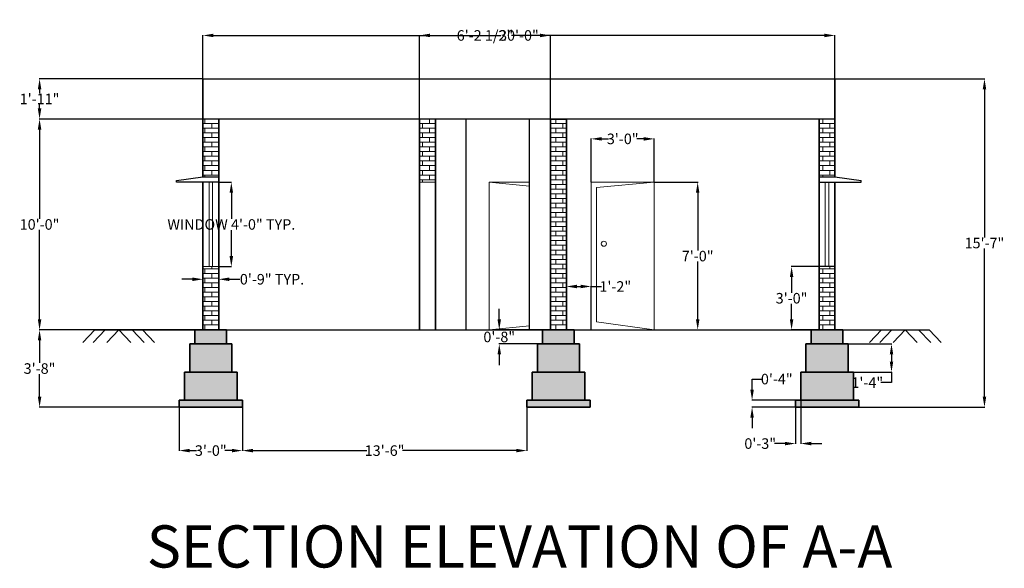
# Model space of a CAD drawing. Units: inches. Extents: x 94 to 277359, y -289541 to 1081.
# Tile 4 of 5: x 740 to 1300, y 353 to 665. Entities that reach past the tile are written whole.
import ezdxf

# ---------------------------------------------------------------- set-up
doc = ezdxf.new("R2010")
doc.units = ezdxf.units.IN
doc.header["$MEASUREMENT"] = 0
doc.layers.get('Defpoints').update_dxf_attribs({"color": 255})
for name, color, linetype, lineweight in [('A-ANNO-DIMS', 2, 'Continuous', 18), ('A-ANNO-TEXT', 7, 'Continuous', 30), ('A-DOOR', 4, 'Continuous', 18), ('A-ELEV', 7, 'Continuous', 25), ('A-ROOF', 7, 'Continuous', 30), ('A-SECT', 7, 'Continuous', 35), ('A-WALL-PATT', 252, 'Continuous', 13), ('C-TOPO', 8, 'Continuous', 25), ('S-FNDN', 7, 'Continuous', 35), ('S-FNDN-PATT', 252, 'Continuous', 13), ('window', 13, 'Continuous', 18)]:
    doc.layers.add(name, color=color, linetype=linetype, lineweight=lineweight)
doc.styles.get("Standard").update_dxf_attribs({"font": 'arial.ttf'})
doc.dimstyles.get("Standard").update_dxf_attribs({"dimtxt": 6, "dimasz": 6, "dimexe": 0.18, "dimexo": 0.0625, "dimgap": 0.09, "dimtad": 0, "dimtih": 1, "dimtoh": 1, "dimdec": 1, "dimzin": 0, "dimdsep": 46, "dimlunit": 3, "dimtxsty": 'Standard', "dimcen": 0.09, "dimadec": 0, "dimazin": 0, "dimtfac": 1, "dimtdec": 1, "dimtofl": 0, "dimtmove": 0, "dimatfit": 3, "dimfxl": 1, "dimtolj": 1, "dimtzin": 0, "dimarcsym": 0})
pattern_1 = [(50, (-239.0183, 16.959), (7.172602, -0.627521), [0.75, -8.25]), (355, (-239.018, 16.959), (-1.387513, 7.52192), [0.6, -6.6]), (100.45144, (-238.4206, 16.907), (5.78509, 6.8944), [0.637402, -7.01142]), (46.1842, (-239.018, 18.959), (10.672413, -1.655193), [1.125, -12.375]), (96.6356, (-238.129, 18.821), (9.34662, 9.741186), [0.9561, -10.51714]), (351.1842, (-239.018, 18.959), (9.34662, 9.741186), [0.9, -9.9]), (21, (-238.0183, 18.459), (5.96907, -4.02619), [0.75, -8.25]), (326, (-238.018, 18.459), (2.433153, 7.2515), [0.6, -6.6]), (71.45144, (-237.521, 18.124), (8.402224, 3.22531), [0.637402, -7.01142]), (37.5, (-239.0183, 16.9592), (0.1215986, 3.3289385), [0, -6.52, 0, -6.7, 0, -6.625]), (7.5, (-239.0183, 16.9592), (2.630695, 3.944117), [0, -3.82, 0, -6.37, 0, -2.525]), (327.5, (-241.2483, 16.9592), (5.3382244, -0.2255487), [0, -2.5, 0, -7.8, 0, -10.35]), (317.5, (-242.2483, 16.9592), (5.831862, 1.00105), [0, -3.25, 0, -5.18, 0, -7.35])]

# ---------------------------------------------------------------- blocks, each defined once
blk = doc.blocks.new('WE')
at = {"layer": 'window'}
for p, q in [((39.8, -77.7), (48.8, -77.7)), ((43.3, -77.7), (43.3, -125.7)), ((45.3, -77.7), (45.3, -125.7)), ((39.8, -125.7), (48.8, -125.7))]:
    blk.add_line(p, q, dxfattribs=at)
blk = doc.blocks.new('GRADE-MARK')
for p, q in [((6.85, 7.09), (0, 0)), ((12.76, 7.09), (5.91, 0)), ((20.39, 7.09), (13.54, 0)), ((20.39, 7.09), (27.24, 0)), ((28.01, 7.09), (34.86, 0)), ((33.93, 7.09), (40.78, 0))]:
    blk.add_line(p, q)
blk = doc.blocks.new('*D33')
at = {"layer": 'A-ANNO-DIMS', "color": 0, "lineweight": -2, "transparency": 16777216}
for p, q in [((853.01, 572.91), (860.33, 572.91)), ((860.15, 566.91), (860.15, 552.1)), ((860.15, 530.91), (860.15, 545.71)), ((853.01, 524.91), (860.33, 524.91))]:
    blk.add_line(p, q, dxfattribs=at)
at = {"layer": 'A-ANNO-DIMS', "color": 0, "transparency": 16777216}
for points in [[(859.15, 566.91), (861.15, 566.91), (860.15, 572.91)], [(859.15, 530.91), (861.15, 530.91), (860.15, 524.91)]]:
    blk.add_solid(points, dxfattribs=at)
at = {"layer": 'Defpoints', "color": 0, "transparency": 16777216}
for p in [(852.95, 572.91), (860.15, 572.91), (852.95, 524.91)]:
    blk.add_point(p, dxfattribs=at)
at = {"layer": 'A-ANNO-DIMS', "color": 0, "transparency": 16777216, "insert": (860.15, 548.91), "char_height": 6, "attachment_point": 5}
blk.add_mtext('\\A1;WINDOW 4\'-0" TYP.', dxfattribs=at)
blk = doc.blocks.new('*D34')
at = {"layer": 'A-ANNO-DIMS', "color": 0, "lineweight": -2, "transparency": 16777216}
for p, q in [((843.95, 524.84), (843.95, 517.53)), ((852.95, 524.84), (852.95, 517.53)), ((837.95, 517.71), (831.95, 517.71)), ((858.95, 517.71), (864.95, 517.71))]:
    blk.add_line(p, q, dxfattribs=at)
at = {"layer": 'A-ANNO-DIMS', "color": 0, "transparency": 16777216}
for points in [[(837.95, 518.71), (837.95, 516.71), (843.95, 517.71)], [(858.95, 518.71), (858.95, 516.71), (852.95, 517.71)]]:
    blk.add_solid(points, dxfattribs=at)
at = {"layer": 'Defpoints', "color": 0, "transparency": 16777216}
for p in [(843.95, 524.91), (852.95, 524.91), (852.95, 517.71)]:
    blk.add_point(p, dxfattribs=at)
at = {"layer": 'A-ANNO-DIMS', "color": 0, "transparency": 16777216, "insert": (883.32, 517.71), "char_height": 6, "attachment_point": 5}
blk.add_mtext('\\A1;0\'-9" TYP.', dxfattribs=at)
blk = doc.blocks.new('*D80')
at = {"layer": 'A-ANNO-DIMS', "color": 0, "lineweight": -2, "transparency": 16777216}
for p, q in [((843.95, 631.84), (843.95, 656.65)), ((849.95, 656.47), (1013.55, 656.47)), ((1197.95, 656.47), (1034.34, 656.47)), ((1203.95, 631.84), (1203.95, 656.65))]:
    blk.add_line(p, q, dxfattribs=at)
at = {"layer": 'A-ANNO-DIMS', "color": 0, "transparency": 16777216}
for points in [[(849.95, 657.47), (849.95, 655.47), (843.95, 656.47)], [(1197.95, 657.47), (1197.95, 655.47), (1203.95, 656.47)]]:
    blk.add_solid(points, dxfattribs=at)
at = {"layer": 'Defpoints', "color": 0, "transparency": 16777216}
for p in [(1203.95, 656.47), (843.95, 631.77), (1203.95, 631.77)]:
    blk.add_point(p, dxfattribs=at)
at = {"layer": 'A-ANNO-DIMS', "color": 0, "transparency": 16777216, "insert": (1023.95, 656.47), "char_height": 6, "attachment_point": 5}
blk.add_mtext('\\A1;30\'-0"', dxfattribs=at)
blk = doc.blocks.new('*D81')
at = {"layer": 'A-ANNO-DIMS', "color": 0, "lineweight": -2, "transparency": 16777216}
for p, q in [((1204.01, 631.77), (1289.27, 631.77)), ((1289.09, 625.77), (1289.09, 541.49)), ((1289.09, 450.91), (1289.09, 535.19)), ((1217.51, 444.91), (1289.27, 444.91))]:
    blk.add_line(p, q, dxfattribs=at)
at = {"layer": 'A-ANNO-DIMS', "color": 0, "transparency": 16777216}
for points in [[(1288.09, 625.77), (1290.09, 625.77), (1289.09, 631.77)], [(1288.09, 450.91), (1290.09, 450.91), (1289.09, 444.91)]]:
    blk.add_solid(points, dxfattribs=at)
at = {"layer": 'Defpoints', "color": 0, "transparency": 16777216}
for p in [(1203.95, 631.77), (1289.09, 631.77), (1217.45, 444.91)]:
    blk.add_point(p, dxfattribs=at)
at = {"layer": 'A-ANNO-DIMS', "color": 0, "transparency": 16777216, "insert": (1289.09, 538.34), "char_height": 6, "attachment_point": 5}
blk.add_mtext('\\A1;15\'-7"', dxfattribs=at)
blk = doc.blocks.new('*D82')
at = {"layer": 'A-ANNO-DIMS', "color": 0, "lineweight": -2, "transparency": 16777216}
for p, q in [((843.89, 608.91), (750.74, 608.91)), ((750.92, 602.91), (750.92, 552.06)), ((750.92, 494.91), (750.92, 545.75)), ((843.89, 488.91), (750.74, 488.91))]:
    blk.add_line(p, q, dxfattribs=at)
at = {"layer": 'A-ANNO-DIMS', "color": 0, "transparency": 16777216}
for points in [[(749.92, 602.91), (751.92, 602.91), (750.92, 608.91)], [(749.92, 494.91), (751.92, 494.91), (750.92, 488.91)]]:
    blk.add_solid(points, dxfattribs=at)
at = {"layer": 'Defpoints', "color": 0, "transparency": 16777216}
for p in [(750.92, 608.91), (843.95, 608.91), (843.95, 488.91)]:
    blk.add_point(p, dxfattribs=at)
at = {"layer": 'A-ANNO-DIMS', "color": 0, "transparency": 16777216, "insert": (750.92, 548.91), "char_height": 6, "attachment_point": 5}
blk.add_mtext('\\A1;10\'-0"', dxfattribs=at)
blk = doc.blocks.new('*D83')
at = {"layer": 'A-ANNO-DIMS', "color": 0, "lineweight": -2, "transparency": 16777216}
for p, q in [((839.39, 488.91), (750.74, 488.91)), ((750.92, 482.91), (750.92, 470.06)), ((750.92, 450.91), (750.92, 463.75)), ((830.39, 444.91), (750.74, 444.91))]:
    blk.add_line(p, q, dxfattribs=at)
at = {"layer": 'A-ANNO-DIMS', "color": 0, "transparency": 16777216}
for points in [[(749.92, 482.91), (751.92, 482.91), (750.92, 488.91)], [(749.92, 450.91), (751.92, 450.91), (750.92, 444.91)]]:
    blk.add_solid(points, dxfattribs=at)
at = {"layer": 'Defpoints', "color": 0, "transparency": 16777216}
for p in [(750.92, 488.91), (839.45, 488.91), (830.45, 444.91)]:
    blk.add_point(p, dxfattribs=at)
at = {"layer": 'A-ANNO-DIMS', "color": 0, "transparency": 16777216, "insert": (750.92, 466.91), "char_height": 6, "attachment_point": 5}
blk.add_mtext('\\A1;3\'-8"', dxfattribs=at)
blk = doc.blocks.new('*D84')
at = {"layer": 'A-ANNO-DIMS', "color": 0, "lineweight": -2, "transparency": 16777216}
for p, q in [((843.89, 631.77), (750.74, 631.77)), ((750.92, 625.77), (750.92, 623.44)), ((750.92, 614.91), (750.92, 617.24)), ((843.89, 608.91), (750.74, 608.91))]:
    blk.add_line(p, q, dxfattribs=at)
at = {"layer": 'A-ANNO-DIMS', "color": 0, "transparency": 16777216}
for points in [[(749.92, 625.77), (751.92, 625.77), (750.92, 631.77)], [(749.92, 614.91), (751.92, 614.91), (750.92, 608.91)]]:
    blk.add_solid(points, dxfattribs=at)
at = {"layer": 'Defpoints', "color": 0, "transparency": 16777216}
for p in [(750.92, 631.77), (843.95, 631.77), (843.95, 608.91)]:
    blk.add_point(p, dxfattribs=at)
at = {"layer": 'A-ANNO-DIMS', "color": 0, "transparency": 16777216, "insert": (750.92, 620.34), "char_height": 6, "attachment_point": 5}
blk.add_mtext('\\A1;1\'-11"', dxfattribs=at)
blk = doc.blocks.new('*D85')
at = {"layer": 'A-ANNO-DIMS', "color": 0, "lineweight": -2, "transparency": 16777216}
for p, q in [((830.45, 444.84), (830.45, 420.03)), ((866.45, 444.84), (866.45, 420.03)), ((836.45, 420.21), (840.39, 420.21)), ((860.45, 420.21), (856.51, 420.21))]:
    blk.add_line(p, q, dxfattribs=at)
at = {"layer": 'A-ANNO-DIMS', "color": 0, "transparency": 16777216}
for points in [[(836.45, 421.21), (836.45, 419.21), (830.45, 420.21)], [(860.45, 421.21), (860.45, 419.21), (866.45, 420.21)]]:
    blk.add_solid(points, dxfattribs=at)
at = {"layer": 'Defpoints', "color": 0, "transparency": 16777216}
for p in [(830.45, 444.91), (866.45, 444.91), (866.45, 420.21)]:
    blk.add_point(p, dxfattribs=at)
at = {"layer": 'A-ANNO-DIMS', "color": 0, "transparency": 16777216, "insert": (848.45, 420.21), "char_height": 6, "attachment_point": 5}
blk.add_mtext('\\A1;3\'-0"', dxfattribs=at)
blk = doc.blocks.new('*D86')
at = {"layer": 'A-ANNO-DIMS', "color": 0, "lineweight": -2, "transparency": 16777216}
for p, q in [((866.45, 444.84), (866.45, 420.03)), ((1028.45, 444.84), (1028.45, 420.03)), ((872.45, 420.21), (937.33, 420.21)), ((1022.45, 420.21), (957.56, 420.21))]:
    blk.add_line(p, q, dxfattribs=at)
at = {"layer": 'A-ANNO-DIMS', "color": 0, "transparency": 16777216}
for points in [[(872.45, 421.21), (872.45, 419.21), (866.45, 420.21)], [(1022.45, 421.21), (1022.45, 419.21), (1028.45, 420.21)]]:
    blk.add_solid(points, dxfattribs=at)
at = {"layer": 'Defpoints', "color": 0, "transparency": 16777216}
for p in [(866.45, 444.91), (1028.45, 444.91), (1028.45, 420.21)]:
    blk.add_point(p, dxfattribs=at)
at = {"layer": 'A-ANNO-DIMS', "color": 0, "transparency": 16777216, "insert": (947.45, 420.21), "char_height": 6, "attachment_point": 5}
blk.add_mtext('\\A1;13\'-6"', dxfattribs=at)
blk = doc.blocks.new('*D87')
at = {"layer": 'A-ANNO-DIMS', "color": 0, "lineweight": -2, "transparency": 16777216}
for p, q in [((967.32, 608.97), (967.32, 656.65)), ((973.32, 656.47), (989.56, 656.47)), ((1035.95, 656.47), (1019.7, 656.47)), ((1041.95, 608.97), (1041.95, 656.65))]:
    blk.add_line(p, q, dxfattribs=at)
at = {"layer": 'A-ANNO-DIMS', "color": 0, "transparency": 16777216}
for points in [[(973.32, 657.47), (973.32, 655.47), (967.32, 656.47)], [(1035.95, 657.47), (1035.95, 655.47), (1041.95, 656.47)]]:
    blk.add_solid(points, dxfattribs=at)
at = {"layer": 'Defpoints', "color": 0, "transparency": 16777216}
for p in [(1041.95, 656.47), (967.32, 608.91), (1041.95, 608.91)]:
    blk.add_point(p, dxfattribs=at)
at = {"layer": 'A-ANNO-DIMS', "color": 0, "transparency": 16777216, "insert": (1004.63, 656.47), "char_height": 6, "attachment_point": 5}
blk.add_mtext('\\A1;6\'-2 1/2"', dxfattribs=at)
blk = doc.blocks.new('*D88')
at = {"layer": 'A-ANNO-DIMS', "color": 0, "lineweight": -2, "transparency": 16777216}
for p, q in [((1101.13, 572.91), (1125.94, 572.91)), ((1125.76, 566.91), (1125.76, 534.06)), ((1125.76, 494.91), (1125.76, 527.75)), ((1101.13, 488.91), (1125.94, 488.91))]:
    blk.add_line(p, q, dxfattribs=at)
at = {"layer": 'A-ANNO-DIMS', "color": 0, "transparency": 16777216}
for points in [[(1124.76, 566.91), (1126.76, 566.91), (1125.76, 572.91)], [(1124.76, 494.91), (1126.76, 494.91), (1125.76, 488.91)]]:
    blk.add_solid(points, dxfattribs=at)
at = {"layer": 'Defpoints', "color": 0, "transparency": 16777216}
for p in [(1101.06, 572.91), (1101.06, 488.91), (1125.76, 488.91)]:
    blk.add_point(p, dxfattribs=at)
at = {"layer": 'A-ANNO-DIMS', "color": 0, "transparency": 16777216, "insert": (1125.76, 530.91), "char_height": 6, "attachment_point": 5}
blk.add_mtext('\\A1;7\'-0"', dxfattribs=at)
blk = doc.blocks.new('*D89')
at = {"layer": 'A-ANNO-DIMS', "color": 0, "lineweight": -2, "transparency": 16777216}
for p, q in [((1065.06, 572.97), (1065.06, 597.79)), ((1071.06, 597.61), (1075, 597.61)), ((1095.06, 597.61), (1091.13, 597.61)), ((1101.06, 572.97), (1101.06, 597.79))]:
    blk.add_line(p, q, dxfattribs=at)
at = {"layer": 'A-ANNO-DIMS', "color": 0, "transparency": 16777216}
for points in [[(1071.06, 598.61), (1071.06, 596.61), (1065.06, 597.61)], [(1095.06, 598.61), (1095.06, 596.61), (1101.06, 597.61)]]:
    blk.add_solid(points, dxfattribs=at)
at = {"layer": 'Defpoints', "color": 0, "transparency": 16777216}
for p in [(1101.06, 597.61), (1065.06, 572.91), (1101.06, 572.91)]:
    blk.add_point(p, dxfattribs=at)
at = {"layer": 'A-ANNO-DIMS', "color": 0, "transparency": 16777216, "insert": (1083.06, 597.61), "char_height": 6, "attachment_point": 5}
blk.add_mtext('\\A1;3\'-0"', dxfattribs=at)
blk = doc.blocks.new('*D90')
at = {"layer": 'A-ANNO-DIMS', "color": 0, "lineweight": -2, "transparency": 16777216}
for p, q in [((1203.89, 524.91), (1179.07, 524.91)), ((1179.25, 518.91), (1179.25, 510.06)), ((1179.25, 494.91), (1179.25, 503.75)), ((1203.89, 488.91), (1179.07, 488.91))]:
    blk.add_line(p, q, dxfattribs=at)
at = {"layer": 'A-ANNO-DIMS', "color": 0, "transparency": 16777216}
for points in [[(1178.25, 518.91), (1180.25, 518.91), (1179.25, 524.91)], [(1178.25, 494.91), (1180.25, 494.91), (1179.25, 488.91)]]:
    blk.add_solid(points, dxfattribs=at)
at = {"layer": 'Defpoints', "color": 0, "transparency": 16777216}
for p in [(1179.25, 524.91), (1203.95, 524.91), (1203.95, 488.91)]:
    blk.add_point(p, dxfattribs=at)
at = {"layer": 'A-ANNO-DIMS', "color": 0, "transparency": 16777216, "insert": (1179.25, 506.91), "char_height": 6, "attachment_point": 5}
blk.add_mtext('\\A1;3\'-0"', dxfattribs=at)
blk = doc.blocks.new('*D91')
at = {"layer": 'A-ANNO-DIMS', "color": 0, "lineweight": -2, "transparency": 16777216}
for p, q in [((1050.95, 488.97), (1050.95, 513.79)), ((1056.95, 513.61), (1059.06, 513.61)), ((1065.06, 488.97), (1065.06, 513.79)), ((1065.06, 513.61), (1071.06, 513.61))]:
    blk.add_line(p, q, dxfattribs=at)
at = {"layer": 'A-ANNO-DIMS', "color": 0, "transparency": 16777216}
for points in [[(1056.95, 514.61), (1056.95, 512.61), (1050.95, 513.61)], [(1059.06, 514.61), (1059.06, 512.61), (1065.06, 513.61)]]:
    blk.add_solid(points, dxfattribs=at)
at = {"layer": 'Defpoints', "color": 0, "transparency": 16777216}
for p in [(1065.06, 513.61), (1050.95, 488.91), (1065.06, 488.91)]:
    blk.add_point(p, dxfattribs=at)
at = {"layer": 'A-ANNO-DIMS', "color": 0, "transparency": 16777216, "insert": (1078.85, 513.61), "char_height": 6, "attachment_point": 5}
blk.add_mtext('\\A1;1\'-2"', dxfattribs=at)
blk = doc.blocks.new('*D92')
at = {"layer": 'A-ANNO-DIMS', "color": 0, "lineweight": -2, "transparency": 16777216}
for p, q in [((1012.747749, 494.905028), (1012.747749, 500.905028)), ((1037.385249, 488.905028), (1012.567749, 488.905028)), ((1037.385249, 480.905028), (1012.567749, 480.905028)), ((1012.747749, 474.905028), (1012.747749, 468.905028))]:
    blk.add_line(p, q, dxfattribs=at)
at = {"layer": 'A-ANNO-DIMS', "color": 0, "transparency": 16777216}
for points in [[(1011.747749, 494.905028), (1013.747749, 494.905028), (1012.747749, 488.905028)], [(1011.747749, 474.905028), (1013.747749, 474.905028), (1012.747749, 480.905028)]]:
    blk.add_solid(points, dxfattribs=at)
at = {"layer": 'Defpoints', "color": 0, "transparency": 16777216}
for p in [(1012.747749, 488.905028), (1037.447749, 488.905028), (1037.447749, 480.905028)]:
    blk.add_point(p, dxfattribs=at)
at = {"layer": 'A-ANNO-DIMS', "color": 0, "transparency": 16777216, "insert": (1012.747749, 484.905028), "char_height": 6, "attachment_point": 5}
blk.add_mtext('\\A1;0\'-8"', dxfattribs=at)
blk = doc.blocks.new('*D93')
at = {"layer": 'A-ANNO-DIMS', "color": 0, "lineweight": -2, "transparency": 16777216}
for p, q in [((1211.51, 480.91), (1236.33, 480.91)), ((1236.15, 474.91), (1236.15, 470.91)), ((1211.51, 464.91), (1236.33, 464.91)), ((1236.15, 464.91), (1236.15, 458.91)), ((1236.15, 458.91), (1230.15, 458.91))]:
    blk.add_line(p, q, dxfattribs=at)
at = {"layer": 'A-ANNO-DIMS', "color": 0, "transparency": 16777216}
for points in [[(1235.15, 474.91), (1237.15, 474.91), (1236.15, 480.91)], [(1235.15, 470.91), (1237.15, 470.91), (1236.15, 464.91)]]:
    blk.add_solid(points, dxfattribs=at)
at = {"layer": 'Defpoints', "color": 0, "transparency": 16777216}
for p in [(1211.45, 480.91), (1211.45, 464.91), (1236.15, 464.91)]:
    blk.add_point(p, dxfattribs=at)
at = {"layer": 'A-ANNO-DIMS', "color": 0, "transparency": 16777216, "insert": (1222.37, 458.91), "char_height": 6, "attachment_point": 5}
blk.add_mtext('\\A1;1\'-4"', dxfattribs=at)
blk = doc.blocks.new('*D94')
at = {"layer": 'A-ANNO-DIMS', "color": 0, "lineweight": -2, "transparency": 16777216}
for p, q in [((1181.45, 448.84), (1181.45, 424.03)), ((1184.45, 448.84), (1184.45, 424.03)), ((1175.45, 424.21), (1169.45, 424.21)), ((1190.45, 424.21), (1196.45, 424.21))]:
    blk.add_line(p, q, dxfattribs=at)
at = {"layer": 'A-ANNO-DIMS', "color": 0, "transparency": 16777216}
for points in [[(1175.45, 425.21), (1175.45, 423.21), (1181.45, 424.21)], [(1190.45, 425.21), (1190.45, 423.21), (1184.45, 424.21)]]:
    blk.add_solid(points, dxfattribs=at)
at = {"layer": 'Defpoints', "color": 0, "transparency": 16777216}
for p in [(1181.45, 448.91), (1184.45, 448.91), (1181.45, 424.21)]:
    blk.add_point(p, dxfattribs=at)
at = {"layer": 'A-ANNO-DIMS', "color": 0, "transparency": 16777216, "insert": (1161.38, 424.21), "char_height": 6, "attachment_point": 5}
blk.add_mtext('\\A1;0\'-3"', dxfattribs=at)
blk = doc.blocks.new('*D95')
at = {"layer": 'A-ANNO-DIMS', "color": 0, "lineweight": -2, "transparency": 16777216}
for p, q in [((1156.75, 454.91), (1156.75, 460.91)), ((1156.75, 460.91), (1162.75, 460.91)), ((1181.39, 448.91), (1156.57, 448.91)), ((1181.39, 444.91), (1156.57, 444.91)), ((1156.75, 438.91), (1156.75, 432.91))]:
    blk.add_line(p, q, dxfattribs=at)
at = {"layer": 'A-ANNO-DIMS', "color": 0, "transparency": 16777216}
for points in [[(1155.75, 454.91), (1157.75, 454.91), (1156.75, 448.91)], [(1155.75, 438.91), (1157.75, 438.91), (1156.75, 444.91)]]:
    blk.add_solid(points, dxfattribs=at)
at = {"layer": 'Defpoints', "color": 0, "transparency": 16777216}
for p in [(1156.75, 448.91), (1181.45, 448.91), (1181.45, 444.91)]:
    blk.add_point(p, dxfattribs=at)
at = {"layer": 'A-ANNO-DIMS', "color": 0, "transparency": 16777216, "insert": (1170.81, 460.91), "char_height": 6, "attachment_point": 5}
blk.add_mtext('\\A1;0\'-4"', dxfattribs=at)

msp = doc.modelspace()

# ---------------------------------------------------------------- hatches: boundary and pattern name
at = {"layer": 'A-WALL-PATT'}
h = msp.add_hatch(dxfattribs=at)
h.set_pattern_fill('AR-BRSTD', color=256)
h.set_pattern_definition([(0, (-239.0183, 16.9592), (0, 2.667), []), (90, (-239.0183, 16.9592), (-4, 2.667), [2.667, -2.667])])
h.paths.add_polyline_path([(852.95, 608.91), (843.95, 608.91), (843.95, 575.91), (852.95, 575.91)])
h.paths.add_polyline_path([(852.95, 524.91), (843.95, 524.91), (843.95, 488.91), (848.45, 488.91), (852.95, 488.91)])
h.paths.add_polyline_path([(976.4, 608.91), (967.32, 608.91), (967.32, 572.91), (976.4, 572.91)])
h.paths.add_polyline_path([(1041.95, 488.91), (1046.45, 488.91), (1050.95, 488.91), (1050.95, 608.91), (1041.95, 608.91)])
h.paths.add_polyline_path([(1194.95, 575.91), (1203.95, 575.91), (1203.95, 608.91), (1194.95, 608.91)])
h.paths.add_polyline_path([(1203.95, 524.91), (1194.95, 524.91), (1194.95, 488.91), (1199.45, 488.91), (1203.95, 488.91)])
at = {"layer": 'S-FNDN-PATT'}
h = msp.add_hatch(dxfattribs=at)
h.set_pattern_fill('AR-CONC', color=256)
h.set_pattern_definition(pattern_1)
h.paths.add_polyline_path([(848.45, 480.91), (857.45, 480.91), (857.45, 488.91), (848.45, 488.91), (839.45, 488.91), (839.45, 480.91)])
h.paths.add_polyline_path([(1055.45, 480.91), (1055.45, 488.91), (1046.45, 488.91), (1037.45, 488.91), (1037.45, 480.91), (1046.45, 480.91)])
h.paths.add_polyline_path([(1199.45, 480.91), (1208.45, 480.91), (1208.45, 488.91), (1199.45, 488.91), (1190.45, 488.91), (1190.45, 480.91)])
h = msp.add_hatch(dxfattribs=at)
h.set_pattern_fill('ANSI33', color=256, scale=10)
h.set_pattern_definition([(45, (-239.0183, 16.9592), (-1.767767, 1.767767), []), (45, (-237.2506, 16.9592), (-1.767767, 1.767767), [1.25, -0.625])])
h.paths.add_polyline_path([(863.45, 464.91), (848.45, 464.91), (836.45, 464.91), (833.45, 464.91), (833.45, 448.91), (848.45, 448.91), (863.45, 448.91)])
h.paths.add_polyline_path([(860.45, 480.91), (848.45, 480.91), (839.45, 480.91), (836.45, 480.91), (836.45, 464.91), (848.45, 464.91), (860.45, 464.91)])
h.paths.add_polyline_path([(1061.45, 464.91), (1046.45, 464.91), (1034.45, 464.91), (1031.45, 464.91), (1031.45, 448.91), (1046.45, 448.91), (1061.45, 448.91)])
h.paths.add_polyline_path([(1058.45, 480.91), (1046.45, 480.91), (1037.45, 480.91), (1034.45, 480.91), (1034.45, 464.91), (1046.45, 464.91), (1058.45, 464.91)])
h.paths.add_polyline_path([(1214.45, 464.91), (1199.45, 464.91), (1187.45, 464.91), (1184.45, 464.91), (1184.45, 448.91), (1199.45, 448.91), (1214.45, 448.91)])
h.paths.add_polyline_path([(1211.45, 480.91), (1199.45, 480.91), (1190.45, 480.91), (1187.45, 480.91), (1187.45, 464.91), (1199.45, 464.91), (1211.45, 464.91)])
h = msp.add_hatch(dxfattribs=at)
h.set_pattern_fill('AR-CONC', color=256)
h.set_pattern_definition(pattern_1)
h.paths.add_polyline_path([(866.45, 444.91), (866.45, 448.91), (848.45, 448.91), (833.45, 448.91), (830.45, 448.91), (830.45, 444.91)])
h.paths.add_polyline_path([(1064.45, 448.91), (1046.45, 448.91), (1031.45, 448.91), (1028.45, 448.91), (1028.45, 444.91), (1064.45, 444.91)])
h.paths.add_polyline_path([(1217.45, 444.91), (1217.45, 448.91), (1199.45, 448.91), (1184.45, 448.91), (1181.45, 448.91), (1181.45, 444.91)])

# ---------------------------------------------------------------- linework, layer by layer
at = {"layer": 'A-DOOR'}
for p, q in [((976.4, 572.91), (967.32, 572.91)), ((976.4, 488.91), (976.4, 572.91)), ((1006.95, 488.91), (1006.95, 572.91)), ((1006.95, 572.91), (1029.95, 572.91)), ((1006.95, 572.91), (1029.95, 570.71)), ((1065.06, 488.91), (1065.06, 572.91)), ((1065.06, 572.91), (1101.06, 572.91)), ((1101.06, 572.91), (1068.16, 569.94)), ((1101.06, 572.91), (1101.06, 488.91)), ((1068.16, 569.94), (1068.16, 493.45)), ((1006.95, 488.91), (1029.95, 491.24)), ((1068.16, 493.45), (1101.06, 488.91))]:
    msp.add_line(p, q, dxfattribs=at)
msp.add_circle((1072.34, 537.94), 1.47, dxfattribs=at)
at = {"layer": 'A-ELEV'}
for p, q in [((993.95, 488.91), (993.95, 608.91)), ((1029.95, 488.91), (1029.95, 608.91))]:
    msp.add_line(p, q, dxfattribs=at)
at = {"layer": 'A-ROOF'}
for p, q in [((843.95, 631.77), (1203.95, 631.77)), ((1203.95, 608.91), (843.95, 608.91)), ((828.95, 573.91), (843.95, 575.91)), ((828.95, 572.91), (828.95, 573.91)), ((852.95, 572.91), (828.95, 572.91)), ((843.95, 575.91), (852.95, 575.91)), ((1194.95, 572.91), (1194.95, 575.91)), ((1194.95, 575.91), (1203.95, 575.91)), ((1194.95, 572.91), (1218.95, 572.91)), ((1203.95, 575.91), (1218.95, 573.91)), ((1218.95, 572.91), (1218.95, 573.91))]:
    msp.add_line(p, q, dxfattribs=at)
at = {"layer": 'A-SECT'}
for p, q in [((843.95, 575.91), (843.95, 631.77)), ((1203.95, 575.91), (1203.95, 631.77)), ((852.95, 608.91), (852.95, 488.91)), ((967.32, 488.91), (967.32, 608.91)), ((976.4, 488.91), (976.4, 608.91)), ((1041.95, 488.91), (1041.95, 608.91)), ((1041.95, 608.91), (1050.95, 608.91)), ((1050.95, 608.91), (1050.95, 488.91)), ((1194.95, 488.91), (1194.95, 608.91)), ((843.95, 488.91), (843.95, 572.91)), ((1203.95, 488.91), (1203.95, 572.91)), ((843.95, 488.91), (852.95, 488.91)), ((1041.95, 488.91), (1050.95, 488.91)), ((1194.95, 488.91), (1203.95, 488.91))]:
    msp.add_line(p, q, dxfattribs=at)
at = {"layer": 'C-TOPO'}
msp.add_line((782.46, 488.91), (1257.54, 488.91), dxfattribs=at)
at = {"layer": 'S-FNDN'}
for p, q in [((839.45, 480.91), (839.45, 488.91)), ((839.45, 488.91), (848.45, 488.91)), ((857.45, 488.91), (848.45, 488.91)), ((857.45, 480.91), (857.45, 488.91)), ((1037.45, 480.91), (1037.45, 488.91)), ((1037.45, 488.91), (1046.45, 488.91)), ((1055.45, 488.91), (1046.45, 488.91)), ((1055.45, 480.91), (1055.45, 488.91)), ((1190.45, 480.91), (1190.45, 488.91)), ((1190.45, 488.91), (1199.45, 488.91)), ((1208.45, 488.91), (1199.45, 488.91)), ((1208.45, 480.91), (1208.45, 488.91)), ((836.45, 464.91), (836.45, 480.91)), ((836.45, 480.91), (848.45, 480.91)), ((848.45, 480.91), (839.45, 480.91)), ((860.45, 480.91), (848.45, 480.91)), ((848.45, 480.91), (857.45, 480.91)), ((860.45, 464.91), (860.45, 480.91)), ((1034.45, 464.91), (1034.45, 480.91)), ((1034.45, 480.91), (1046.45, 480.91)), ((1046.45, 480.91), (1037.45, 480.91)), ((1058.45, 480.91), (1046.45, 480.91)), ((1046.45, 480.91), (1055.45, 480.91)), ((1058.45, 464.91), (1058.45, 480.91)), ((1187.45, 464.91), (1187.45, 480.91)), ((1187.45, 480.91), (1199.45, 480.91)), ((1199.45, 480.91), (1190.45, 480.91)), ((1211.45, 480.91), (1199.45, 480.91)), ((1199.45, 480.91), (1208.45, 480.91)), ((1211.45, 464.91), (1211.45, 480.91)), ((833.45, 448.91), (833.45, 464.91)), ((833.45, 464.91), (848.45, 464.91)), ((848.45, 464.91), (836.45, 464.91)), ((863.45, 464.91), (848.45, 464.91)), ((848.45, 464.91), (860.45, 464.91)), ((863.45, 448.91), (863.45, 464.91)), ((1031.45, 448.91), (1031.45, 464.91)), ((1031.45, 464.91), (1046.45, 464.91)), ((1046.45, 464.91), (1034.45, 464.91)), ((1061.45, 464.91), (1046.45, 464.91)), ((1046.45, 464.91), (1058.45, 464.91)), ((1061.45, 448.91), (1061.45, 464.91)), ((1184.45, 448.91), (1184.45, 464.91)), ((1184.45, 464.91), (1199.45, 464.91)), ((1199.45, 464.91), (1187.45, 464.91)), ((1214.45, 464.91), (1199.45, 464.91)), ((1199.45, 464.91), (1211.45, 464.91)), ((1214.45, 448.91), (1214.45, 464.91)), ((830.45, 444.91), (830.45, 448.91)), ((830.45, 448.91), (848.45, 448.91)), ((848.45, 448.91), (833.45, 448.91)), ((866.45, 448.91), (848.45, 448.91)), ((848.45, 448.91), (863.45, 448.91)), ((866.45, 444.91), (866.45, 448.91)), ((1028.45, 444.91), (1028.45, 448.91)), ((1028.45, 448.91), (1046.45, 448.91)), ((1046.45, 448.91), (1031.45, 448.91)), ((1064.45, 448.91), (1046.45, 448.91)), ((1046.45, 448.91), (1061.45, 448.91)), ((1064.45, 444.91), (1064.45, 448.91)), ((1181.45, 444.91), (1181.45, 448.91)), ((1181.45, 448.91), (1199.45, 448.91)), ((1199.45, 448.91), (1184.45, 448.91)), ((1217.45, 448.91), (1199.45, 448.91)), ((1199.45, 448.91), (1214.45, 448.91)), ((1217.45, 444.91), (1217.45, 448.91)), ((830.45, 444.91), (866.45, 444.91)), ((866.45, 444.91), (830.45, 444.91)), ((1028.45, 444.91), (1064.45, 444.91)), ((1064.45, 444.91), (1028.45, 444.91)), ((1181.45, 444.91), (1217.45, 444.91)), ((1217.45, 444.91), (1181.45, 444.91))]:
    msp.add_line(p, q, dxfattribs=at)

# ---------------------------------------------------------------- block references
at = {"layer": 'C-TOPO'}
for p in [(775.62, 481.81), (1223.61, 481.81)]:
    msp.add_blockref('GRADE-MARK', p, dxfattribs=at)
at = {"layer": 'window'}
for p in [(804.15, 650.61), (1155.15, 650.61)]:
    msp.add_blockref('WE', p, dxfattribs=at)

# ---------------------------------------------------------------- texts
at = {"layer": 'A-ANNO-TEXT', "insert": (1024.31, 377.66), "char_height": 24, "attachment_point": 2}
msp.add_mtext_dynamic_manual_height_columns('SECTION ELEVATION OF A-A ', width=589.888, gutter_width=1, heights=[0], dxfattribs=at)

# ---------------------------------------------------------------- dimensions: what is measured, and where the dimension line sits
at = {"layer": 'A-ANNO-DIMS'}
for base, p1, p2, picture, middle in [((1041.95, 656.47), (967.32, 608.91), (1041.95, 608.91), '*D87', (1004.63, 656.47)), ((1203.95, 656.47), (843.95, 631.77), (1203.95, 631.77), '*D80', (1023.95, 656.47)), ((1101.06, 597.61), (1065.06, 572.91), (1101.06, 572.91), '*D89', (1083.06, 597.61)), ((1065.06, 513.61), (1050.95, 488.91), (1065.06, 488.91), '*D91', (1078.85, 513.61)), ((866.45, 420.21), (830.45, 444.91), (866.45, 444.91), '*D85', (848.45, 420.21)), ((1028.45, 420.21), (866.45, 444.91), (1028.45, 444.91), '*D86', (947.45, 420.21))]:
    dim = msp.add_linear_dim(base=base, p1=p1, p2=p2, dimstyle='Standard', override={"dimdec": 1, "dimlfac": 1, "dimrnd": 0, "dimzin": 1, "dimdsep": 46, "dimlunit": 4, "dimfrac": 2}, dxfattribs=at)
    dim.commit()
    dim.dimension.update_dxf_attribs({"geometry": picture, "text_midpoint": middle})
for base, p1, p2, angle, picture, middle in [((750.92, 631.77), (843.95, 608.91), (843.95, 631.77), 90, '*D84', (750.92, 620.34)), ((1289.09, 631.77), (1217.45, 444.91), (1203.95, 631.77), 90, '*D81', (1289.09, 538.34)), ((750.92, 608.91), (843.95, 488.91), (843.95, 608.91), 90, '*D82', (750.92, 548.91)), ((1125.76, 488.91), (1101.06, 572.91), (1101.06, 488.91), 270, '*D88', (1125.76, 530.91)), ((1179.25, 524.91), (1203.95, 488.91), (1203.95, 524.91), 90, '*D90', (1179.25, 506.91)), ((1012.75, 488.91), (1037.45, 480.91), (1037.45, 488.91), 90, '*D92', (1012.75, 484.91)), ((750.92, 488.91), (830.45, 444.91), (839.45, 488.91), 90, '*D83', (750.92, 466.91)), ((1236.15, 464.91), (1211.45, 480.91), (1211.45, 464.91), 270, '*D93', (1222.37, 458.91)), ((1156.75, 448.91), (1181.45, 444.91), (1181.45, 448.91), 90, '*D95', (1170.81, 460.91)), ((1181.45, 424.21), (1184.45, 448.91), (1181.45, 448.91), 180, '*D94', (1161.38, 424.21))]:
    dim = msp.add_linear_dim(base=base, p1=p1, p2=p2, angle=angle, dimstyle='Standard', override={"dimdec": 1, "dimlfac": 1, "dimrnd": 0, "dimzin": 1, "dimdsep": 46, "dimlunit": 4, "dimfrac": 2}, dxfattribs=at)
    dim.commit()
    dim.dimension.update_dxf_attribs({"geometry": picture, "text_midpoint": middle})
dim = msp.add_linear_dim(base=(860.15, 572.91), p1=(852.95, 524.91), p2=(852.95, 572.91), angle=90, text='WINDOW <> TYP.', dimstyle='Standard', override={"dimdec": 1, "dimlfac": 1, "dimrnd": 0, "dimzin": 1, "dimdsep": 46, "dimlunit": 4, "dimfrac": 2}, dxfattribs=at)
dim.commit()
dim.dimension.update_dxf_attribs({"geometry": '*D33', "text_midpoint": (860.15, 548.91)})
dim = msp.add_linear_dim(base=(852.95, 517.71), p1=(843.95, 524.91), p2=(852.95, 524.91), text='<> TYP.', dimstyle='Standard', override={"dimdec": 1, "dimlfac": 1, "dimrnd": 0, "dimzin": 1, "dimdsep": 46, "dimlunit": 4, "dimfrac": 2}, dxfattribs=at)
dim.commit()
dim.dimension.update_dxf_attribs({"geometry": '*D34', "text_midpoint": (883.32, 517.71)})

doc.saveas('drawing.dxf')
